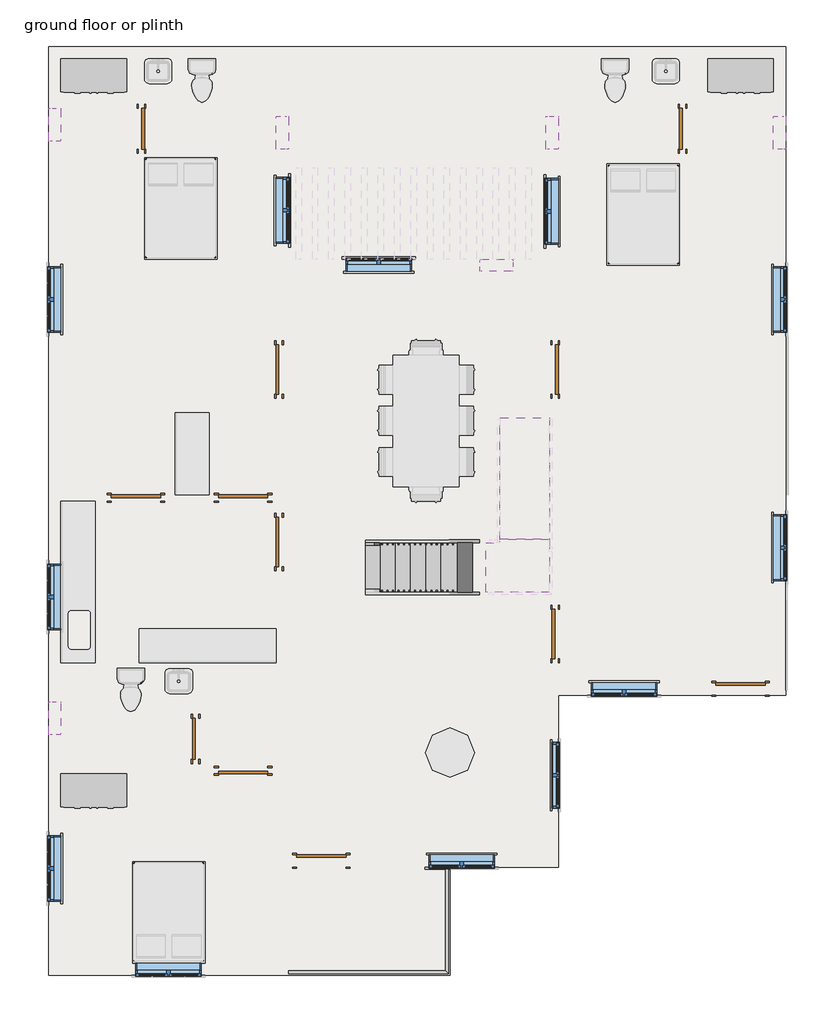
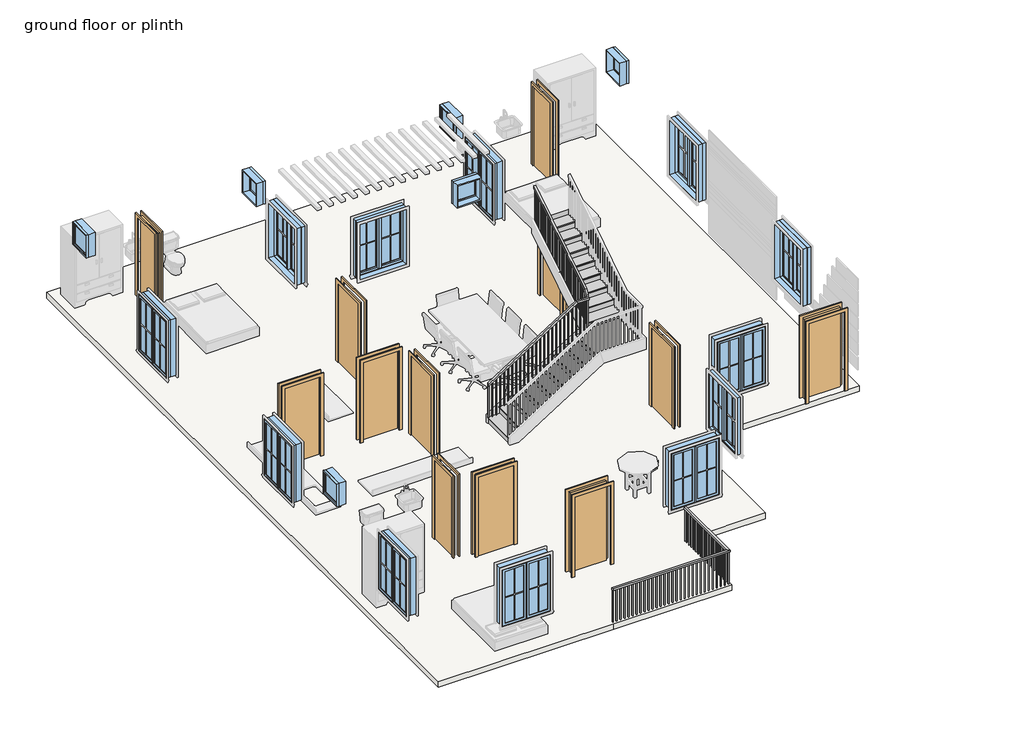
# One storey, part 1 of 3: 18 windows, 12 doors, 2 railings, 2 slabs, 2 stair flights.
# Revit data of these elements (continued)
# Element 34 (IfcWindow, "Window-Casement-Double : 48\" x 60\"") (continued)
#   Window Inset = 0' - 0"
#   Interior Wall Closure = 0' - 2 1/4"
#   Frame Extension = 0' - 0 1/4"
#   Exterior Wall Closure = 0' - 1 1/4"
#   Interior Trim Visibility = yes
#   Exterior Trim Visibility = yes
#   Phase Created = New Construction
#   Materials on its faces: "Wood - Stained", "Glass", "Clad - White"
# Element 35 (IfcWindow, "Window-Casement-Double : 48\" x 60\"")
#   Mark = "18"
#   Window Inset = 0' - 0"
#   Interior Wall Closure = 0' - 2 1/4"
#   Frame Extension = 0' - 0 1/4"
#   Exterior Wall Closure = 0' - 1 1/4"
#   Interior Trim Visibility = yes
#   Exterior Trim Visibility = yes
#   Phase Created = New Construction
#   Materials on its faces: "Wood - Stained", "Glass", "Clad - White"
# Element 36 (IfcWindow, "Window-Casement-Double : 48\" x 60\"")
#   Mark = "9"
#   Window Inset = 0' - 0"
#   Interior Wall Closure = 0' - 2 1/4"
#   Frame Extension = 0' - 0 1/4"
#   Exterior Wall Closure = 0' - 1 1/4"
#   Interior Trim Visibility = yes
#   Exterior Trim Visibility = yes
#   Phase Created = New Construction
#   Materials on its faces: "Wood - Stained", "Glass", "Clad - White"
# Materials
#   "Door - Panel": class "Wood", colour RGB 210 159 95, transparency 0, Cost = 0
#   "Door - Frame": colour RGB 118 70 51, transparency 0, Cost = 0
#   "Concrete, Cast-in-Place gray": class "Concrete", colour RGB 192 192 192, transparency 0, Description = "Cast-in-place concrete", Cost = 0
#   "Glass": class "Glass", colour RGB 0 128 192, transparency 0.75, Description = "Soda Lime Glass", Cost = 0
#   "Sash": class "Wood", colour RGB 224 178 126, transparency 0, Cost = 0
#   "Wood - Stained": class "Wood", colour RGB 224 178 126, transparency 0, Cost = 0
#   "Clad - White": class "Wood", colour RGB 242 242 238, transparency 0, Cost = 0
